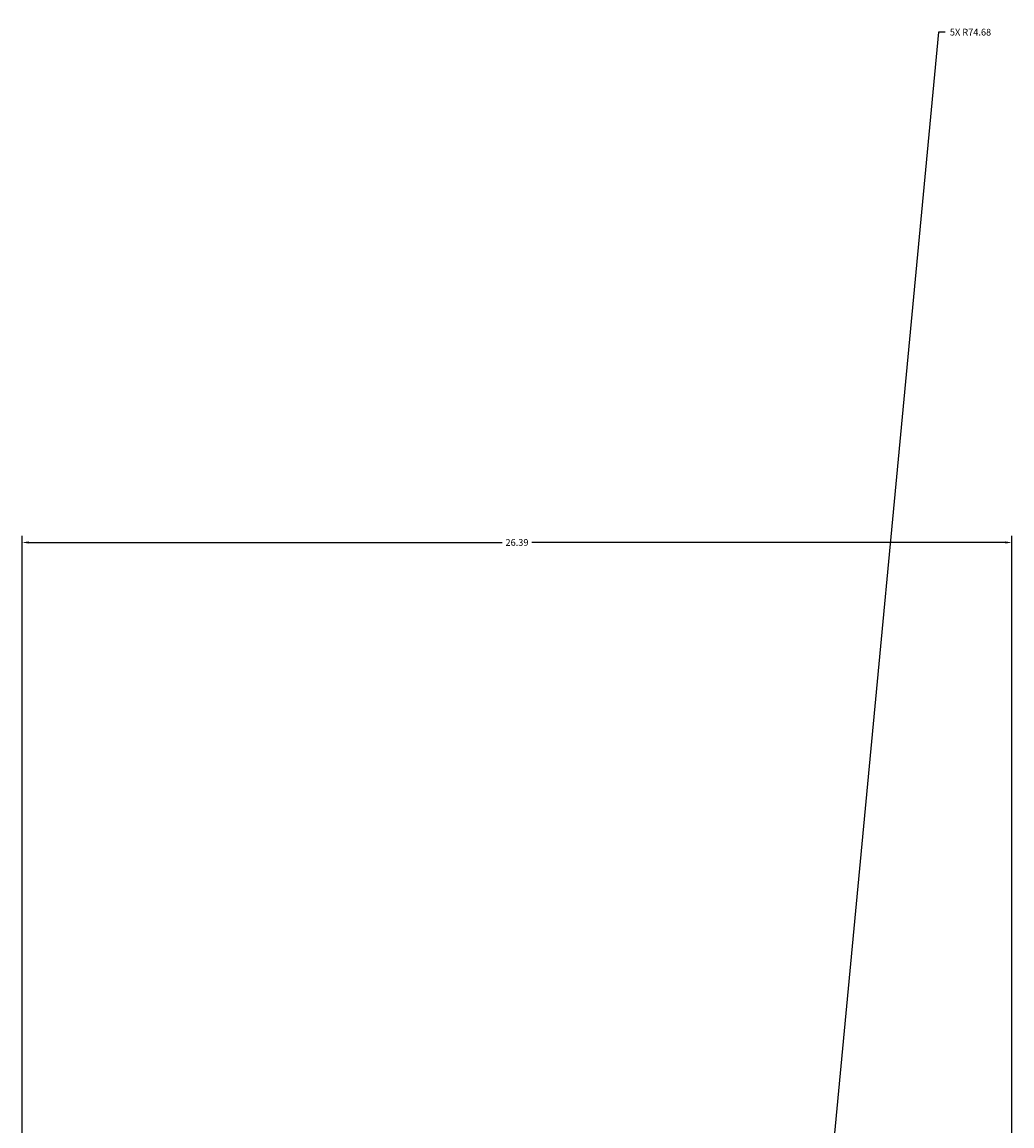
# Model space of a CAD drawing. Units: inches. Extents: x -99 to 284, y -92 to 134.
# Tile 11 of 16: x 19 to 45, y 105 to 134. Entities that reach past the tile are written whole.
import ezdxf

# ---------------------------------------------------------------- set-up
doc = ezdxf.new("R2010")
doc.units = ezdxf.units.IN
doc.header["$MEASUREMENT"] = 0
doc.layers.add('M-DIMS', color=2, linetype='Continuous', lineweight=18)
doc.styles.get("Standard").update_dxf_attribs({"font": 'arial.ttf'})
doc.dimstyles.get("Standard").update_dxf_attribs({"dimtxt": 0.18, "dimasz": 0.18, "dimexe": 0.18, "dimexo": 0.0625, "dimgap": 0.09, "dimtad": 0, "dimtih": 1, "dimtoh": 1, "dimdec": 4, "dimzin": 0, "dimdsep": 46, "dimtxsty": 'Standard', "dimcen": 0.09, "dimadec": 0, "dimazin": 0, "dimtfac": 1, "dimtdec": 4, "dimtofl": 0, "dimtmove": 0, "dimatfit": 3, "dimfxl": 1, "dimtolj": 1, "dimtzin": 0, "dimarcsym": 0})

# ---------------------------------------------------------------- blocks, each defined once
blk = doc.blocks.new('*D10')
at = {"layer": 'Defpoints', "color": 0, "transparency": 16777216}
for p in [(45.172, 120.204), (18.781, 88.36), (45.172, 88.36)]:
    blk.add_point(p, dxfattribs=at)
at = {"layer": 'M-DIMS', "color": 0, "lineweight": -2, "transparency": 16777216}
for p, q in [((18.781, 88.422), (18.781, 120.384)), ((18.961, 120.204), (31.581, 120.204)), ((44.992, 120.204), (32.372, 120.204)), ((45.172, 88.422), (45.172, 120.384))]:
    blk.add_line(p, q, dxfattribs=at)
at = {"layer": 'M-DIMS', "color": 0, "transparency": 16777216}
for points in [[(18.961, 120.234), (18.961, 120.174), (18.781, 120.204)], [(44.992, 120.234), (44.992, 120.174), (45.172, 120.204)]]:
    blk.add_solid(points, dxfattribs=at)
at = {"layer": 'M-DIMS', "color": 0, "transparency": 16777216, "insert": (31.976, 120.204), "char_height": 0.18, "attachment_point": 5}
blk.add_mtext('\\A1;26.39', dxfattribs=at)
blk = doc.blocks.new('*D22')
at = {"layer": 'Defpoints', "color": 0, "transparency": 16777216}
for p in [(39, 89.203), (31.976, 14.854)]:
    blk.add_point(p, dxfattribs=at)
at = {"layer": 'M-DIMS', "color": 0, "lineweight": -2, "transparency": 16777216}
for p, q in [((43.215, 133.813), (39.017, 89.383)), ((43.395, 133.813), (43.215, 133.813)), ((31.886, 14.854), (32.066, 14.854)), ((31.976, 14.764), (31.976, 14.944))]:
    blk.add_line(p, q, dxfattribs=at)
at = {"layer": 'M-DIMS', "color": 0, "transparency": 16777216}
blk.add_solid([(38.987, 89.385), (39.047, 89.38), (39, 89.203)], dxfattribs=at)
at = {"layer": 'M-DIMS', "color": 0, "transparency": 16777216, "insert": (44.068, 133.813), "char_height": 0.18, "attachment_point": 5}
blk.add_mtext('\\A1;5X R74.68', dxfattribs=at)

msp = doc.modelspace()

# ---------------------------------------------------------------- dimensions: what is measured, and where the dimension line sits
at = {"layer": 'M-DIMS'}
dim = msp.add_radius_dim(center=(31.9765, 14.8539), mpoint=(39.0003, 89.2035), text='5X <>', dimstyle='Standard', override={"dimdec": 2, "dimlfac": 1, "dimrnd": 0, "dimzin": 0, "dimdsep": 46, "dimlunit": 2}, dxfattribs=at)
dim.commit()
dim.dimension.update_dxf_attribs({"geometry": '*D22', "text_midpoint": (44.068, 133.8132), "dimtype": 164})
dim = msp.add_linear_dim(base=(45.1717, 120.2039), p1=(18.7812, 88.3595), p2=(45.1717, 88.3595), dimstyle='Standard', override={"dimdec": 2, "dimlfac": 1, "dimrnd": 0, "dimzin": 0, "dimdsep": 46, "dimlunit": 2}, dxfattribs=at)
dim.commit()
dim.dimension.update_dxf_attribs({"geometry": '*D10', "text_midpoint": (31.9765, 120.2039)})

doc.saveas('drawing.dxf')
